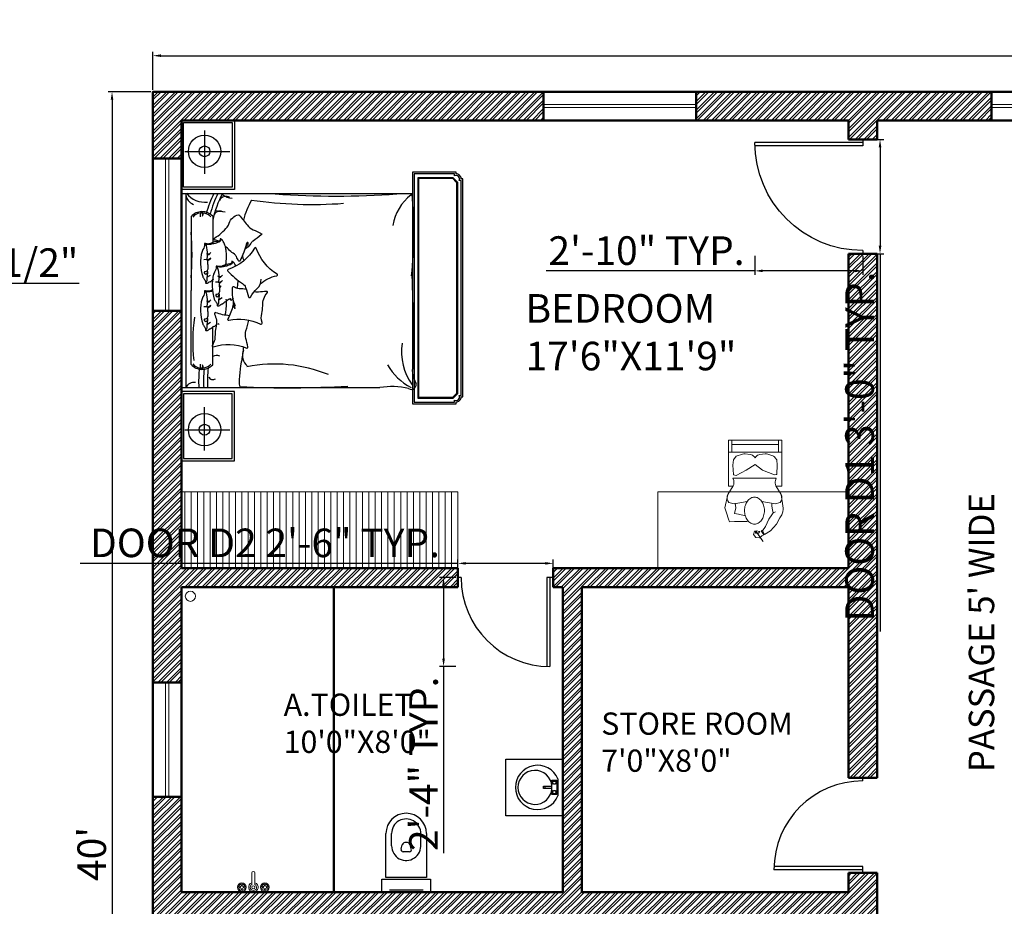
# Model space of a CAD drawing. Units: inches. Extents: x 3590 to 5167, y 65 to 1917.
# Tile 27 of 100: x 4378 to 4688, y 1549 to 1829. Entities that reach past the tile are written whole.
import ezdxf

# ---------------------------------------------------------------- set-up
doc = ezdxf.new("R2010")
doc.units = ezdxf.units.IN
for name, color, linetype, lineweight in [('A-ANNO-DIMS', 2, 'Continuous', 18), ('A-AREA-IDEN', 7, 'Continuous', 18), ('A-DOOR', 3, 'Continuous', 25), ('A-FLOR-FIXT', 8, 'Continuous', 18), ('A-FURN', 21, 'Continuous', 18), ('A-GLAZ', 4, 'Continuous', 18), ('A-WALL', 7, 'Continuous', 50), ('A-WALL-PATT', 251, 'Continuous', 13)]:
    doc.layers.add(name, color=color, linetype=linetype, lineweight=lineweight)
for name, color, linetype in [('FUR', 42, 'Continuous'), ('HA-FUR', 8, 'Continuous'), ('HA-P', 8, 'Continuous'), ('SAN', 5, 'Continuous'), ('SANTEH', 7, 'Continuous'), ('wood', 26, 'Continuous')]:
    doc.layers.add(name, color=color, linetype=linetype)
doc.styles.get("Standard").update_dxf_attribs({"font": 'arial.ttf'})
doc.dimstyles.new('ISO-25', dxfattribs={"dimtxt": 9, "dimasz": 2.5, "dimexe": 1.25, "dimexo": 0.625, "dimtad": 1, "dimdec": 1, "dimlunit": 3, "dimtxsty": 'Standard', "dimcen": 2.5, "dimadec": 0, "dimazin": 0, "dimtfac": 1, "dimtdec": 1, "dimtmove": 0, "dimatfit": 3, "dimfxl": 1, "dimarcsym": 0})

# ---------------------------------------------------------------- blocks, each defined once
blk = doc.blocks.new('*D101')
at = {"layer": 'A-ANNO-DIMS', "color": 0, "lineweight": -2, "transparency": 16777216}
for p, q in [((4420.27, 1806.62), (4420.27, 1818.61)), ((4422.77, 1817.36), (5077.77, 1817.36)), ((5080.27, 1806.62), (5080.27, 1818.61))]:
    blk.add_line(p, q, dxfattribs=at)
at = {"layer": 'A-ANNO-DIMS', "color": 0, "transparency": 16777216}
for points in [[(4422.77, 1817.78), (4422.77, 1816.95), (4420.27, 1817.36)], [(5077.77, 1817.78), (5077.77, 1816.95), (5080.27, 1817.36)]]:
    blk.add_solid(points, dxfattribs=at)
at = {"layer": 'Defpoints', "color": 0, "transparency": 16777216}
for p in [(5080.27, 1817.36), (4420.27, 1806), (5080.27, 1806)]:
    blk.add_point(p, dxfattribs=at)
at = {"layer": 'A-ANNO-DIMS', "color": 0, "transparency": 16777216, "insert": (4750.27, 1822.57), "char_height": 9, "attachment_point": 5}
blk.add_mtext("55'", dxfattribs=at)
blk = doc.blocks.new('*D102')
at = {"layer": 'A-ANNO-DIMS', "color": 0, "lineweight": -2, "transparency": 16777216}
for p, q in [((4419.65, 1806), (4406.15, 1806)), ((4407.4, 1803.5), (4407.4, 1328.5)), ((4419.65, 1326), (4406.15, 1326))]:
    blk.add_line(p, q, dxfattribs=at)
at = {"layer": 'A-ANNO-DIMS', "color": 0, "transparency": 16777216}
for points in [[(4406.98, 1803.5), (4407.82, 1803.5), (4407.4, 1806)], [(4406.98, 1328.5), (4407.82, 1328.5), (4407.4, 1326)]]:
    blk.add_solid(points, dxfattribs=at)
at = {"layer": 'Defpoints', "color": 0, "transparency": 16777216}
for p in [(4420.27, 1806), (4407.4, 1326), (4420.27, 1326)]:
    blk.add_point(p, dxfattribs=at)
at = {"layer": 'A-ANNO-DIMS', "color": 0, "transparency": 16777216, "insert": (4402.18, 1566), "char_height": 9, "attachment_point": 5, "rotation": 90}
blk.add_mtext("40'", dxfattribs=at)
blk = doc.blocks.new('D1')
for p, q in [((1, 0), (1, 34)), ((2, 0), (2, 33.99)), ((0, 0), (2, 0)), ((35, 0), (36, 0))]:
    blk.add_line(p, q)
at = {"ltscale": 0.5}
blk.add_arc((1, 0), 34, 0, 90, dxfattribs=at)
blk = doc.blocks.new('D2')
for p, q in [((1, 0), (1, 28)), ((2, 0), (2, 27.98)), ((0, 0), (2, 0)), ((29, 0), (30, 0))]:
    blk.add_line(p, q)
at = {"ltscale": 0.5}
blk.add_arc((1, 0), 28, 0, 90, dxfattribs=at)
blk = doc.blocks.new('Faucet - Bathroom top')
for p, q in [((-4.107, 0.125), (-4.375, 0.125)), ((-3.75, 0.4788), (-3.75, 0.75)), ((-3.5, 0.482), (-3.5, 0.75)), ((-3.1461, 0.125), (-2.875, 0.125)), ((3.143, 0.125), (2.875, 0.125)), ((3.5, 0.4788), (3.5, 0.75)), ((3.75, 0.482), (3.75, 0.75)), ((4.1039, 0.125), (4.375, 0.125)), ((-4.1039, -0.125), (-4.375, -0.125)), ((-3.75, -0.4821), (-3.75, -0.75)), ((-3.5, -0.4789), (-3.5, -0.75)), ((-3.143, -0.125), (-2.875, -0.125)), ((-0.5, -0.8639), (-0.5, -4.5)), ((0.5, -4.5), (0.5, -0.8631)), ((3.1461, -0.125), (2.875, -0.125)), ((3.5, -0.4821), (3.5, -0.75)), ((3.75, -0.4789), (3.75, -0.75)), ((4.107, -0.125), (4.375, -0.125))]:
    blk.add_line(p, q)
for centre, radius in [((-3.625, 0), 1.375), ((-4.625, 0), 0.2795), ((-3.625, 0), 0.5), ((-3.625, 1), 0.2795), ((-2.625, 0), 0.2795), ((0, 0), 0.5), ((3.625, 0), 1.375), ((2.625, 0), 0.2795), ((3.625, 0), 0.5), ((3.625, 1), 0.2795), ((4.625, 0), 0.2795), ((-3.625, -1), 0.2795), ((3.625, -1), 0.2795)]:
    blk.add_circle(centre, radius)
for centre, radius, start, end in [((-3.625, 0), 1, 105.2407, 164.2093), ((-3.625, 0), 1, 16.44125, 74.07887), ((0, 0), 1.5, 289.6514, 250.3603), ((0, 0), 1, 300.3431, 239.7554), ((3.625, 0), 1, 106.12, 164.0884), ((3.625, 0), 1, 16.23422, 73.90469), ((-3.625, 0), 1, 196.2342, 253.9047), ((-3.625, 0), 1, 286.12, 344.0884), ((3.625, 0), 1, 196.4413, 254.0789), ((3.625, 0), 1, 285.2407, 344.2093), ((0, -4.5), 0.5, 180, 0)]:
    blk.add_arc(centre, radius, start, end)
blk = doc.blocks.new('y3')
at = {"layer": 'SANTEH', "ltscale": 5}
for p, q in [((37.5, 130.7), (37.5, 520.7)), ((87.5, 410.7), (87.5, 520.7)), ((346.6, 426.1), (347.5, 520.7)), ((397.5, 520.7), (397.5, 130.7)), ((171.9, 384.5), (181.1, 421.3)), ((244.3, 357.8), (190.7, 357.8)), ((263.1, 384.5), (253.9, 421.3)), ((397.5, 130.7), (37.5, 130.7)), ((67.5, 20.7), (367.5, 20.7))]:
    blk.add_line(p, q, dxfattribs=at)
blk.add_lwpolyline([(0, 115), (435, 115), (435, 0), (0, 0), (0, 115)], dxfattribs=at)
for centre, radius, start, end in [((217.5, 520.7), 180, 0, 180), ((217.5, 520.7), 130, 359.15795, 180), ((217.5, 399.9), 42.2, 30.52342, 149.47658), ((217.5, 410.7), 130, 180, 5.98548), ((190.7, 377.8), 20, 160.50385, 270), ((244.3, 377.8), 20, 270, 19.49615)]:
    blk.add_arc(centre, radius, start, end, dxfattribs=at)
blk = doc.blocks.new('r11')
at = {"layer": 'SANTEH', "ltscale": 5}
for p, q in [((0, 0), (600, 0)), ((0, -600), (0, 0)), ((600, 0), (600, -600)), ((210, -50), (390, -50)), ((210, -50), (210, -50)), ((224, -63), (376, -63)), ((224, -113), (224, -63)), ((233, -79), (249, -69)), ((233, -98), (233, -79)), ((249, -107), (233, -98)), ((249, -69), (266, -79)), ((266, -98), (249, -107)), ((266, -79), (266, -98)), ((334, -79), (351, -69)), ((334, -98), (334, -79)), ((351, -107), (334, -98)), ((351, -69), (367, -79)), ((367, -98), (351, -107)), ((367, -79), (367, -98)), ((376, -63), (376, -113)), ((376, -113), (224, -113)), ((288, -202), (288, -113)), ((312, -184), (288, -184)), ((312, -202), (288, -202)), ((312, -113), (312, -202)), ((600, -600), (0, -600))]:
    blk.add_line(p, q, dxfattribs=at)
for centre, radius, start, end in [((300, -266), 234, 112.5, 67.5), ((300, -293), 180, 93.8183, 86.1817)]:
    blk.add_arc(centre, radius, start, end, dxfattribs=at)
blk = doc.blocks.new('A$C0A42580C')
at = {"layer": 'SAN'}
for p, q in [((0.2873, 0.0301), (0.2873, 0.4484)), ((2.8678, 0.0301), (2.8678, 0.4484)), ((0.0949, 0.2135), (0.4958, 0.2135)), ((3.0601, 0.2135), (2.6592, 0.2135))]:
    blk.add_line(p, q, dxfattribs=at)
for centre, radius in [((0.2873, 0.2135), 0.15), ((2.8678, 0.2135), 0.15), ((0.2873, 0.2135), 0.05), ((2.8678, 0.2135), 0.05)]:
    blk.add_circle(centre, radius, dxfattribs=at)
at = {"layer": 'wood'}
for p, q in [((0.6775, 0.8851), (0.6775, 2.1392)), ((2.4775, 0.8016), (2.4775, 1.838)), ((2.4775, 0), (2.4775, 0.8016)), ((1.6633, 0.3438), (1.6434, 0.3761)), ((0.888, 0.289), (1.1327, 0.289)), ((1.5, 0.3423), (1.5016, 0.3142)), ((2.267, 0.289), (1.9163, 0.289)), ((1.2906, 0.2348), (1.2921, 0.2067)), ((1.4538, 0.2362), (1.434, 0.2685)), ((1.7287, 0.2348), (1.7302, 0.2067)), ((1.8919, 0.2362), (1.8721, 0.2685)), ((0.6775, 0.039), (2.4775, 0.039)), ((0.8909, 0.089), (1.5775, 0.089)), ((2.2642, 0.089), (1.5775, 0.089)), ((0.6775, 0), (2.4775, 0))]:
    blk.add_line(p, q, dxfattribs=at)
blk.add_lwpolyline([(0.6775, 0), (0.6775, 0.8851)], dxfattribs=at)
for points in [[(1.516, 0.7294, -0.128392), (1.4401, 0.8834, 0.70791), (1.427, 0.8863, -0.16964), (1.1848, 0.6919, 0.664036), (1.184, 0.6776, -0.184649), (1.3819, 0.4332, 0.662242), (1.3969, 0.4309, 0.078539), (1.5137, 0.5669, -0.1736), (1.5484, 0.5947, -0.02159), (1.6357, 0.6205, 0.697276), (1.6379, 0.6405, -0.093019), (1.5606, 0.699, 0.216632), (1.4719, 0.7371, -2.511293)], [(1.1211, 0.3454, 0.032543), (1.1095, 0.3091, -0.658965), (1.0917, 0.3063, 0.074753), (0.9887, 0.4234, 0.100988), (0.953, 0.4429, -0.270711), (0.8753, 0.5273, -0.276825), (0.8775, 0.5337, -0.014937), (0.9701, 0.6081, 0.134834), (1.0135, 0.6643, -0.023706), (1.0474, 0.7372, -0.664036), (1.0616, 0.7394, -0.035987), (1.119, 0.6627, 0.118631), (1.1415, 0.6412, -0.132738), (1.1955, 0.5864)], [(1.6795, 0.4818, 0.263265), (1.7191, 0.4839, -0.026108), (1.743, 0.4973, 0.027613), (1.7137, 0.4764, -0.089259), (1.8403, 0.429, 0.662242), (1.8528, 0.4376, -0.162037), (1.8882, 0.732, 0.676499), (1.8733, 0.748, -0.160513), (1.7901, 0.7439, 0.07473), (1.7202, 0.7523, -0.187721), (1.5966, 0.7963, 0.70791), (1.5851, 0.7895, -0.010003), (1.5921, 0.7143, -0.07079), (1.5891, 0.6719, 0.099539)], [(1.1759, 0.5928, 0.013884), (1.1549, 0.6131, 0.174178), (1.1437, 0.6177, 0.104076), (1.1358, 0.6165, 0.389829), (1.1324, 0.6097, 0.296089), (1.1415, 0.6019, -0.036701), (1.1572, 0.5985, -0.040547), (1.3022, 0.543, -0.70791), (1.3021, 0.5296, -0.016811), (1.2631, 0.5085, 0.11866), (1.2414, 0.4904, -0.048791), (1.1649, 0.4055, 0.103757)], [(1.5674, 0.601, 0.057807), (1.5606, 0.5339, -0.173425), (1.5457, 0.49, 0.589988), (1.5538, 0.4706, 0.137312), (1.7236, 0.4985, 0.137312)], [(1.8113, 0.4446, -0.069098), (1.7831, 0.3187, 0.658965), (1.7961, 0.3062, -0.049789), (1.8516, 0.3234, -0.103757), (1.8905, 0.3233, 0.055725), (2.0203, 0.3103, -0.11866), (2.0478, 0.304, 0.016811), (2.0881, 0.2856, 0.70791), (2.0989, 0.2936, -0.16964), (2.1104, 0.604, 0.664036), (2.1001, 0.6139, 0.023706), (2.0214, 0.597, -0.134834), (1.9505, 0.5976, 0.012748), (1.8522, 0.6228)], [(1.3107, 0.4764, 0.145733), (1.3069, 0.4677, 0.488583), (1.3089, 0.4657, -0.012138), (1.3131, 0.4661, -0.125673), (1.3213, 0.4646, -0.750706)], [(1.3153, 0.4751, -0.274893), (1.3379, 0.4529, 0.051436), (1.3468, 0.4293, -0.086628), (1.3532, 0.4078, 0.040196), (1.3593, 0.3772, -0.184744), (1.3556, 0.3344, -2.554464)], [(1.317, 0.4683, -0.060098), (1.3283, 0.4571, -0.16247), (1.3313, 0.4487, 0.120018), (1.3493, 0.3815, -0.060072), (1.3541, 0.3695, -0.13107), (1.3541, 0.3395, -0.024415), (1.3534, 0.3373, 0.070398), (1.3503, 0.3233, 0.528689), (1.3524, 0.3216, -0.069388), (1.3557, 0.3222, -0.158233), (1.4075, 0.3065, 0.085461), (1.4255, 0.2981, 0.147196), (1.6571, 0.3041, 0.10985), (1.6823, 0.3191, -0.179095), (1.7126, 0.3319, -2.318897)], [(1.1013, 0.3688, 0.145733), (1.0975, 0.3601, 0.488583), (1.0995, 0.3581, -0.012138), (1.1036, 0.3585, -0.125673), (1.1119, 0.357, -0.750706)], [(1.1059, 0.3675, -0.274893), (1.1285, 0.3453, 0.051436), (1.1373, 0.3217, -0.086628), (1.1438, 0.3003, 0.040196), (1.1499, 0.2696, -0.184744), (1.1462, 0.2269, -2.554464)], [(1.4359, 0.3803, -0.198519), (1.452, 0.3494, 0.826402), (1.4558, 0.349, 0.095956), (1.4561, 0.3528, 0.242899), (1.4461, 0.3686, -17.523452)], [(1.5447, 0.3525, -0.083557), (1.507, 0.3546, 0.203162), (1.4851, 0.3792, -0.208037), (1.5043, 0.3409, 0.124669), (1.4432, 0.3469, 0.965934)], [(1.5394, 0.3688, 0.145733), (1.5356, 0.3601, 0.488583), (1.5376, 0.3581, -0.012138), (1.5418, 0.3585, -0.125673), (1.55, 0.357, -0.750706)], [(1.1076, 0.3607, -0.060098), (1.1189, 0.3495, -0.16247), (1.1219, 0.3411, 0.120018), (1.1399, 0.2739, -0.060072), (1.1447, 0.2619, -0.13107), (1.1447, 0.2319, -0.024415), (1.144, 0.2297, 0.070398), (1.1409, 0.2157, 0.528689), (1.143, 0.2141, -0.069388), (1.1463, 0.2146, -0.158233), (1.1981, 0.1989, 0.085461), (1.2161, 0.1905, 0.147196), (1.4477, 0.1965, 0.10985), (1.4728, 0.2115, -0.179095), (1.5032, 0.2244, -2.318897)], [(1.3509, 0.3219, -0.117141), (1.3688, 0.335, -0.025084), (1.4533, 0.348, 0.033691)], [(1.5447, 0.3525, -0.008229), (1.5728, 0.3519, 0.033691)], [(1.5721, 0.286, 0.022869), (1.578, 0.2739, -0.060072), (1.5828, 0.2619, -0.13107), (1.5828, 0.2319, -0.024415), (1.5821, 0.2297, 0.070398), (1.579, 0.2157, 0.528689), (1.5811, 0.2141, -0.069388), (1.5844, 0.2146, -0.158233), (1.6362, 0.1989, 0.085461), (1.6542, 0.1905, 0.147196), (1.8858, 0.1965, 0.10985), (1.911, 0.2115, -0.179095), (1.9413, 0.2244, -2.318897)], [(1.5728, 0.3519, -0.46905), (1.6152, 0.321, 0.420988), (1.62, 0.3169, 0.857652), (1.6221, 0.3484, 0.548526)], [(1.5838, 0.2873, 0.023398), (1.588, 0.2696, -0.184744), (1.5843, 0.2269, -2.554464)], [(1.603, 0.3451, -0.099719), (1.6221, 0.3484, 0.102691)], [(1.6214, 0.3487, -0.010168), (1.6558, 0.3447, 0.033691), (1.6907, 0.3423, -0.220869), (1.7148, 0.3311, -0.288972)], [(1.1415, 0.2143, -0.117141), (1.1594, 0.2274, -0.025084), (1.2439, 0.2405, 0.033691)], [(1.2265, 0.2728, -0.198519), (1.2426, 0.2418, 0.826402), (1.2463, 0.2415, 0.095956), (1.2467, 0.2452, 0.242899), (1.2366, 0.2611, -17.523452)], [(1.3353, 0.2449, -0.083557), (1.2976, 0.247, 0.203162), (1.2757, 0.2717, -0.208037), (1.2948, 0.2333, 0.124669), (1.2338, 0.2393, 0.965934)], [(1.3353, 0.2449, -0.008229), (1.3633, 0.2443, 0.033691)], [(1.3633, 0.2443, -0.46905), (1.4058, 0.2134, 0.420988), (1.4106, 0.2093, 0.857652), (1.4127, 0.2408, 0.548526)], [(1.3936, 0.2375, -0.099719), (1.4127, 0.2408, 0.102691)], [(1.412, 0.2411, -0.010168), (1.4464, 0.2371, 0.033691), (1.4812, 0.2348, -0.220869), (1.5054, 0.2235, -0.288972)], [(1.5796, 0.2143, -0.117141), (1.5975, 0.2274, -0.025084), (1.682, 0.2405, 0.033691)], [(1.6646, 0.2728, -0.198519), (1.6807, 0.2418, 0.826402), (1.6845, 0.2415, 0.095956), (1.6848, 0.2452, 0.242899), (1.6748, 0.2611, -17.523452)], [(1.7734, 0.2449, -0.083557), (1.7357, 0.247, 0.203162), (1.7138, 0.2717, -0.208037), (1.733, 0.2333, 0.124669), (1.6719, 0.2393, 0.965934)], [(1.7734, 0.2449, -0.008229), (1.8015, 0.2443, 0.033691)], [(1.8015, 0.2443, -0.46905), (1.8439, 0.2134, 0.420988), (1.8487, 0.2093, 0.857652), (1.8508, 0.2408, 0.548526)], [(1.8317, 0.2375, -0.099719), (1.8508, 0.2408, 0.102691)], [(1.8501, 0.2411, -0.010168), (1.8845, 0.2371, 0.033691), (1.9193, 0.2348, -0.220869), (1.9435, 0.2235, -0.288972)]]:
    blk.add_lwpolyline(points, format="xyb", dxfattribs=at)
for points in [[(0.64, 0), (0, 0), (0, 0.49), (0.64, 0.49)], [(0.62, 0.02), (0.02, 0.02), (0.02, 0.47), (0.62, 0.47)], [(2.515, 0), (3.155, 0), (3.155, 0.49), (2.515, 0.49)], [(2.535, 0.02), (3.135, 0.02), (3.135, 0.47), (2.535, 0.47)]]:
    blk.add_lwpolyline(points, close=True, dxfattribs=at)
for centre, radius, start, end in [((1.0344, -2.14), 4.292, 84.56078, 94.7164), ((1.0494, 2.4026), 0.4515, 217.47941, 260.35986), ((2.0208, -11.0786), 13.2288, 88.75549, 92.51133), ((2.1491, 2.5471), 0.5083, 260.65485, 306.44155), ((2.3125, 2.3833), 0.2443, 254.1515, 300.95574), ((2.0168, 2.3573), 0.5127, 299.08175, 333.44367), ((2.4501, 2.1309), 0.0445, 324.18954, 118.92203), ((3.1371, 1.9502), 0.669, 166.6404, 189.65708), ((-7.0839, 1.4328), 7.7858, 355.84817, 4.15183), ((-3.167, 1.2143), 3.9465, 351.77286, 4.18386), ((-7.2439, 0.9937), 9.7233, 357.34474, 3.23068), ((3.5803, 0.8622), 1.3213, 157.81295, 191.15154), ((1.1611, 1.4181), 0.8768, 241.21362, 254.41879), ((1.2583, 0.6364), 0.0695, 238.58923, 301.92671), ((1.7861, -2.1601), 2.7557, 80.89877, 83.46656), ((2.181, 0.6859), 0.1221, 247.37754, 321.13165), ((2.4192, 1.3819), 0.8461, 255.77539, 273.25587), ((0.5904, 0.4689), 0.13, 317.38218, 359.70393), ((1.3546, 0.4469), 0.0529, 114.21284, 146.15395), ((2.6126, -2.3504), 3.1201, 113.83178, 114.21284), ((1.4714, 0.0722), 0.4528, 80.62397, 88.74059), ((1.4035, -0.3388), 0.8693, 79.71489, 80.62397), ((1.6301, 0.4539), 0.0342, 31.14095, 54.95422), ((1.6709, 0.4489), 0.0156, 131.9623, 212.08127), ((1.5664, 0.4154), 0.1086, 24.20989, 31.14095), ((1.6627, 0.4587), 0.00309, 275.52245, 24.20989), ((1.1611, 1.3191), 1.0568, 242.76671, 257.10398), ((0.7723, 0.4131), 0.0674, 147.68233, 245.79865), ((0.0312, 0.4583), 0.8174, 350.42368, 356.2506), ((0.9021, 0.3562), 0.0605, 155.8342, 254.41058), ((1.1452, 0.3394), 0.0529, 114.21284, 146.15395), ((2.4032, -2.458), 3.1201, 113.55686, 114.21284), ((1.2046, 0.2912), 0.121, 99.42032, 113.55686), ((1.2774, -0.1478), 0.5659, 95.90379, 99.42032), ((1.2626, -0.005), 0.4223, 88.74059, 95.90379), ((1.2619, -0.0354), 0.4528, 80.62397, 88.74059), ((1.1941, -0.4464), 0.8693, 79.45871, 80.62397), ((1.4207, 0.3463), 0.0342, 31.14095, 54.95422), ((1.6729, 0.4422), 0.0178, 140.41793, 157.63267), ((1.7007, -0.005), 0.4223, 88.74059, 95.90379), ((1.7235, 0.4818), 0.0777, 212.08127, 227.364), ((1.6635, 0.4499), 0.00568, 95.52245, 140.41793), ((1.6391, 0.3902), 0.0469, 17.32618, 47.364), ((1.7106, 0.4125), 0.028, 197.32618, 226.17302), ((1.6431, 0.3422), 0.0695, 26.61764, 46.17302), ((1.8202, 0.431), 0.1287, 206.61764, 215.96192), ((1.7001, -0.0354), 0.4528, 80.62397, 88.74059), ((1.6322, -0.4464), 0.8693, 78.43923, 80.62397), ((1.1611, 1.3191), 1.0937, 243.75553, 254.4906), ((1.1611, 1.2816), 1.0937, 243.75553, 254.38927), ((0.9846, 0.1903), 0.1381, 134.39284, 227.23745), ((1.4614, 0.3413), 0.0156, 131.9623, 212.08127), ((1.4635, 0.3347), 0.0178, 140.41793, 157.63267), ((1.4541, 0.3424), 0.00568, 95.52245, 140.41793), ((1.357, 0.3078), 0.1086, 24.20989, 31.14095), ((1.4533, 0.3511), 0.00309, 275.52245, 24.20989), ((1.5012, 0.305), 0.028, 197.32618, 226.17302), ((1.4337, 0.2347), 0.0695, 26.61764, 46.17302), ((1.715, 0.3349), 0.00379, 207.1817, 328.02977), ((1.6975, 0.3419), 0.023, 350.76434, 35.96192), ((1.7058, 0.3406), 0.0145, 328.02977, 350.76434), ((1.9016, 0.3347), 0.0178, 140.41793, 157.63267), ((1.9522, 0.3743), 0.0777, 212.08127, 227.364), ((1.8922, 0.3424), 0.00568, 95.52245, 140.41793), ((1.8678, 0.2827), 0.0469, 17.32618, 47.364), ((1.9393, 0.305), 0.028, 197.32618, 226.17302), ((1.8718, 0.2347), 0.0695, 26.61764, 46.17302), ((2.2511, 0.3256), 0.071, 155.86842, 211.04513), ((2.1704, 0.1903), 0.1381, 312.76255, 45.60716), ((2.3616, 0.2915), 0.0419, 290.78583, 35.36309), ((0.5293, 0.2241), 0.2307, 309.63048, 4.27465), ((0.8396, 0.185), 0.0112, 314.89662, 45.10338), ((0.8413, 0.1846), 0.0128, 299.47062, 57.44416), ((0.8844, 0.2286), 0.0569, 229.70587, 281.11527), ((0.8802, 0.1371), 0.0592, 81.47786, 123.11925), ((0.8698, 0.1793), 0.0229, 77.14902, 159.1786), ((0.9986, 0.1735), 0.1427, 136.58239, 164.9725), ((1.6108, 0.3235), 0.1287, 206.61764, 215.96192), ((1.5055, 0.2273), 0.00379, 207.1817, 328.02977), ((1.4881, 0.2344), 0.023, 350.76434, 35.96192), ((1.4964, 0.233), 0.0145, 328.02977, 350.76434), ((2.0489, 0.3235), 0.1287, 206.61764, 215.96192), ((1.9436, 0.2273), 0.00379, 207.1817, 328.02977), ((1.9262, 0.2344), 0.023, 350.76434, 35.96192), ((1.9345, 0.233), 0.0145, 328.02977, 350.76434), ((2.2706, 0.2286), 0.0569, 258.88473, 310.29413), ((2.1565, 0.1735), 0.1427, 15.0275, 43.41761), ((2.2749, 0.1371), 0.0592, 56.88075, 98.52214), ((2.2853, 0.1793), 0.0229, 20.8214, 102.85098), ((2.4192, 1.2667), 1.0261, 263.09035, 273.25587), ((2.3138, 0.1846), 0.0128, 122.55584, 240.52938), ((2.3154, 0.185), 0.0112, 134.89662, 225.10338), ((2.4192, 1.2667), 1.0629, 263.94374, 273.25587), ((0.6729, 0.151), 0.1135, 279.23824, 338.73819), ((0.9466, 0.1765), 0.0862, 185.53723, 234.68694), ((1.2481, -2.5919), 2.6893, 85.4722, 94.5278), ((2.0447, 1.7022), 1.5979, 262.13639, 276.48786), ((2.2085, 0.1765), 0.0862, 305.31306, 354.46277), ((2.4192, 1.2218), 1.0629, 263.23622, 273.25587), ((2.508, 0.1152), 0.0792, 169.94668, 248.24015)]:
    blk.add_arc(centre, radius, start, end, dxfattribs=at)
blk = doc.blocks.new('A$C623F1DA0')
at = {"layer": 'FUR'}
blk.add_lwpolyline([(0.628, 2.912, 0.414214), (0.562, 2.978), (0.562, 3), (0, 3), (0, 0), (0.562, 0), (0.562, 0.022, 0.414214), (0.628, 0.088), (0.65, 0.088), (0.65, 2.912)], format="xyb", close=True, dxfattribs=at)
at = {"layer": 'HA-FUR'}
blk.add_lwpolyline([(0.603, 2.892, 0.710288), (0.542, 2.953), (0.542, 2.98), (0.02, 2.98), (0.02, 0.02), (0.542, 0.02), (0.542, 0.047, 0.710288), (0.603, 0.108), (0.63, 0.108), (0.63, 2.892)], format="xyb", close=True, dxfattribs=at)
at = {"layer": 'HA-P'}
for points in [[(0.07, 2.93), (0.521, 2.93), (0.58, 2.871), (0.58, 0.129), (0.521, 0.07), (0.07, 0.07)], [(0.08, 2.92), (0.517, 2.92), (0.57, 2.867), (0.57, 0.133), (0.517, 0.08), (0.08, 0.08)]]:
    blk.add_lwpolyline(points, close=True, dxfattribs=at)
blk = doc.blocks.new('DESK-CHAIR')
for p, q in [((3674.9, 1522.4), (3674.54, 1520.79)), ((3675.51, 1522.74), (3674.9, 1522.4)), ((3680.2, 1521.08), (3677.49, 1522.71)), ((3694.59, 1522.58), (3680.09, 1522.58)), ((3680.09, 1522.58), (3680.09, 1521.15)), ((3694.59, 1505.74), (3694.59, 1522.58)), ((3674.54, 1520.79), (3675.25, 1516.67)), ((3682.6, 1521.15), (3681.85, 1520.9)), ((3682.6, 1521.15), (3682.6, 1507.53)), ((3682.6, 1507.53), (3682.6, 1521.15)), ((3683.49, 1520.07), (3683.66, 1520.91)), ((3685.1, 1517.02), (3683.49, 1520.07)), ((3683.73, 1520.97), (3686.72, 1521.15)), ((3686.72, 1521.15), (3688.33, 1520.97)), ((3688.33, 1520.97), (3689.58, 1520.07)), ((3689.58, 1520.07), (3690.17, 1518.15)), ((3686.89, 1514.16), (3685.1, 1517.02)), ((3690.24, 1517.32), (3690.04, 1515.67)), ((3685.1, 1511.83), (3686.89, 1514.16)), ((3689.31, 1514.37), (3689.04, 1514.16)), ((3689.31, 1513.95), (3689.04, 1514.16)), ((3690.24, 1511), (3690.04, 1512.64)), ((3664.74, 1511.43), (3666.04, 1512.26)), ((3665.07, 1511.29), (3664.74, 1511.43)), ((3664.84, 1511.19), (3666.07, 1511.86)), ((3666.04, 1509.36), (3664.84, 1511.19)), ((3666.04, 1512.26), (3666.24, 1511.79)), ((3666.07, 1511.86), (3667.43, 1510.93)), ((3667.43, 1510.93), (3669.7, 1509.83)), ((3669.7, 1509.83), (3671.06, 1508.9)), ((3674.54, 1507.89), (3675.25, 1512.01)), ((3683.67, 1508.07), (3685.1, 1511.83)), ((3689.78, 1508.89), (3690.17, 1510.17)), ((3668.13, 1507.37), (3666.04, 1509.36)), ((3670.06, 1506.4), (3668.13, 1507.37)), ((3671.06, 1508.9), (3671.66, 1508.47)), ((3671.66, 1508.47), (3671.96, 1507.77)), ((3674.9, 1506.27), (3674.54, 1507.89)), ((3680.2, 1507.6), (3677.49, 1505.97)), ((3680.09, 1507.53), (3680.09, 1505.74)), ((3682.6, 1507.53), (3681.85, 1507.78)), ((3683.8, 1507.4), (3683.67, 1508.07)), ((3683.88, 1507.34), (3686.72, 1507.17)), ((3686.72, 1507.17), (3688.33, 1507.35)), ((3688.33, 1507.35), (3689.03, 1507.86)), ((3677.49, 1505.97), (3673.14, 1505.31)), ((3675.51, 1505.94), (3674.9, 1506.27)), ((3680.09, 1505.74), (3694.59, 1505.74))]:
    blk.add_line(p, q)
for points in [[(3677.49, 1522.71), (3673.28, 1523.65), (3671.67, 1523.12), (3669.7, 1522.58), (3668.81, 1522.22), (3668.99, 1520.61), (3668.99, 1519), (3668.99, 1516.67)], [(3664.74, 1511.43), (3664.42, 1512.05), (3663.77, 1512.78), (3663.87, 1513.9), (3664.88, 1514.67), (3665.92, 1514.37), (3665.9, 1514.02), (3665.32, 1514.02), (3665.3, 1513.1), (3665.82, 1512.66), (3666.07, 1513.84)], [(3671.66, 1508.47), (3672.6, 1508.69), (3673.82, 1508.93), (3674.7, 1508.93)], [(3670.06, 1506.4), (3671.04, 1505.75), (3672.02, 1505.46), (3672.8, 1505.31), (3673.24, 1505.31)]]:
    blk.add_lwpolyline(points)
at = {"const_width": 0.39}
blk.add_lwpolyline([(3666.01, 1513.98), (3662.61, 1511.61)], dxfattribs=at)
for centre, radius, start, end in [((3676.47, 1521), 1.98, 59.0235, 119.0669), ((3681.22, 1522.78), 1.98, 239.0235, 288.4436), ((3683.74, 1520.89), 0.0779, 93.3682, 168.6956), ((3683.74, 1520.89), 0.0779, 93.3682, 168.6956), ((3688.27, 1517.56), 1.98, 352.8785, 17.0946), ((3688.07, 1515.92), 1.98, 308.6739, 352.8785), ((3688.07, 1512.4), 1.98, 7.1215, 51.3261), ((3688.27, 1510.75), 1.98, 342.9054, 7.1215), ((3681.22, 1505.89), 1.98, 71.5564, 120.9765), ((3683.88, 1507.42), 0.0779, 191.3044, 266.6318), ((3687.88, 1509.47), 1.98, 305.5514, 342.9054), ((3676.47, 1507.67), 1.98, 240.9331, 300.9765)]:
    blk.add_arc(centre, radius, start, end)
blk = doc.blocks.new('*D312')
at = {"layer": 'A-ANNO-DIMS', "color": 0, "lineweight": -2, "transparency": 16777216}
for p, q in [((4644.4, 1791), (4650.42, 1791)), ((4649.17, 1788.5), (4649.17, 1757.5)), ((4644.4, 1755), (4650.42, 1755)), ((4649.17, 1755), (4649.17, 1636.06))]:
    blk.add_line(p, q, dxfattribs=at)
at = {"layer": 'A-ANNO-DIMS', "color": 0, "transparency": 16777216}
for points in [[(4648.76, 1788.5), (4649.59, 1788.5), (4649.17, 1791)], [(4648.76, 1757.5), (4649.59, 1757.5), (4649.17, 1755)]]:
    blk.add_solid(points, dxfattribs=at)
at = {"layer": 'Defpoints', "color": 0, "transparency": 16777216}
for p in [(4643.77, 1791), (4643.77, 1755), (4649.17, 1755)]:
    blk.add_point(p, dxfattribs=at)
at = {"layer": 'A-ANNO-DIMS', "color": 0, "transparency": 16777216, "insert": (4643.89, 1694.28), "char_height": 9, "attachment_point": 5, "rotation": 90}
blk.add_mtext('DOOR D1 3\'-0" TYP.', dxfattribs=at)
blk = doc.blocks.new('*D313')
at = {"layer": 'A-ANNO-DIMS', "color": 0, "lineweight": -2, "transparency": 16777216}
for p, q in [((4609.77, 1754.37), (4609.77, 1748.35)), ((4643.77, 1754.37), (4643.77, 1748.35)), ((4609.77, 1749.6), (4544.02, 1749.6)), ((4641.27, 1749.6), (4612.27, 1749.6))]:
    blk.add_line(p, q, dxfattribs=at)
at = {"layer": 'A-ANNO-DIMS', "color": 0, "transparency": 16777216}
for points in [[(4612.27, 1750.02), (4612.27, 1749.18), (4609.77, 1749.6)], [(4641.27, 1750.02), (4641.27, 1749.18), (4643.77, 1749.6)]]:
    blk.add_solid(points, dxfattribs=at)
at = {"layer": 'Defpoints', "color": 0, "transparency": 16777216}
for p in [(4609.77, 1755), (4643.77, 1755), (4609.77, 1749.6)]:
    blk.add_point(p, dxfattribs=at)
at = {"layer": 'A-ANNO-DIMS', "color": 0, "transparency": 16777216, "insert": (4575.65, 1754.82), "char_height": 9, "attachment_point": 5}
blk.add_mtext('2\'-10" TYP.', dxfattribs=at)
blk = doc.blocks.new('*D314')
at = {"layer": 'A-ANNO-DIMS', "color": 0, "lineweight": -2, "transparency": 16777216}
for p, q in [((4516.27, 1653.62), (4516.27, 1658.75)), ((4546.27, 1653.62), (4546.27, 1658.75)), ((4516.27, 1657.5), (4397.34, 1657.5)), ((4543.77, 1657.5), (4518.77, 1657.5))]:
    blk.add_line(p, q, dxfattribs=at)
at = {"layer": 'A-ANNO-DIMS', "color": 0, "transparency": 16777216}
for points in [[(4518.77, 1657.92), (4518.77, 1657.08), (4516.27, 1657.5)], [(4543.77, 1657.92), (4543.77, 1657.08), (4546.27, 1657.5)]]:
    blk.add_solid(points, dxfattribs=at)
at = {"layer": 'Defpoints', "color": 0, "transparency": 16777216}
for p in [(4516.27, 1657.5), (4516.27, 1653), (4546.27, 1653)]:
    blk.add_point(p, dxfattribs=at)
at = {"layer": 'A-ANNO-DIMS', "color": 0, "transparency": 16777216, "insert": (4455.55, 1662.78), "char_height": 9, "attachment_point": 5}
blk.add_mtext('DOOR D2 2\'-6" TYP.', dxfattribs=at)
blk = doc.blocks.new('*D315')
at = {"layer": 'A-ANNO-DIMS', "color": 0, "lineweight": -2, "transparency": 16777216}
for p, q in [((4515.65, 1653), (4510.52, 1653)), ((4511.77, 1650.5), (4511.77, 1627.5)), ((4515.65, 1625), (4510.52, 1625)), ((4511.77, 1625), (4511.77, 1566.24))]:
    blk.add_line(p, q, dxfattribs=at)
at = {"layer": 'A-ANNO-DIMS', "color": 0, "transparency": 16777216}
for points in [[(4511.36, 1650.5), (4512.19, 1650.5), (4511.77, 1653)], [(4511.36, 1627.5), (4512.19, 1627.5), (4511.77, 1625)]]:
    blk.add_solid(points, dxfattribs=at)
at = {"layer": 'Defpoints', "color": 0, "transparency": 16777216}
for p in [(4516.27, 1653), (4511.77, 1625), (4516.27, 1625)]:
    blk.add_point(p, dxfattribs=at)
at = {"layer": 'A-ANNO-DIMS', "color": 0, "transparency": 16777216, "insert": (4506.63, 1594.37), "char_height": 9, "attachment_point": 5, "rotation": 90}
blk.add_mtext('2\'-4" TYP.', dxfattribs=at)
blk = doc.blocks.new('*D320')
at = {"layer": 'A-ANNO-DIMS', "color": 0, "lineweight": -2, "transparency": 16777216}
for p, q in [((4247.49, 1753.73), (4247.49, 1744.5)), ((4304.85, 1753.73), (4304.85, 1744.5)), ((4249.99, 1745.75), (4302.35, 1745.75)), ((4304.85, 1745.75), (4397.07, 1745.75))]:
    blk.add_line(p, q, dxfattribs=at)
at = {"layer": 'A-ANNO-DIMS', "color": 0, "transparency": 16777216}
for points in [[(4249.99, 1746.17), (4249.99, 1745.33), (4247.49, 1745.75)], [(4302.35, 1746.17), (4302.35, 1745.33), (4304.85, 1745.75)]]:
    blk.add_solid(points, dxfattribs=at)
at = {"layer": 'Defpoints', "color": 0, "transparency": 16777216}
for p in [(4247.49, 1754.35), (4304.85, 1754.35), (4304.85, 1745.75)]:
    blk.add_point(p, dxfattribs=at)
at = {"layer": 'A-ANNO-DIMS', "color": 0, "transparency": 16777216, "insert": (4352.21, 1751.03), "char_height": 9, "attachment_point": 5}
blk.add_mtext('PLANT 4\'-9 1/2"', dxfattribs=at)

msp = doc.modelspace()

# ---------------------------------------------------------------- hatches: boundary and pattern name
at = {"layer": 'A-WALL-PATT', "transparency": 33554687}
h = msp.add_hatch(dxfattribs=at)
h.set_pattern_fill('ANSI32', color=256, scale=0.2)
h.paths.add_polyline_path([(4684.27, 1806), (4591.27, 1806), (4591.27, 1797), (4639.27, 1797), (4639.27, 1791), (4648.27, 1791), (4648.27, 1797), (4684.27, 1797)])
h.paths.add_polyline_path([(4543.27, 1806), (4420.27, 1806), (4420.27, 1785), (4429.27, 1785), (4429.27, 1797), (4445.92, 1797), (4543.27, 1797)])
h.paths.add_polyline_path([(4828.27, 1806), (4744.27, 1806), (4744.27, 1797), (4828.27, 1797)])
h.paths.add_polyline_path([(4648.27, 1755), (4639.27, 1755), (4639.27, 1656), (4546.27, 1656), (4546.27, 1650), (4549.27, 1650), (4549.27, 1554), (4429.27, 1554), (4429.27, 1584), (4420.27, 1584), (4420.27, 1539), (4429.27, 1539), (4429.27, 1545), (4639.27, 1545), (4639.27, 1539), (4648.27, 1539), (4648.27, 1560), (4639.27, 1560), (4639.27, 1554), (4555.27, 1554), (4555.27, 1650), (4639.27, 1650), (4639.27, 1590), (4648.27, 1590)])
h.paths.add_polyline_path([(4516.27, 1656), (4429.27, 1656), (4429.27, 1737), (4420.27, 1737), (4420.27, 1620), (4429.27, 1620), (4429.27, 1650), (4516.27, 1650)], flags=17)
h.paths.add_polyline_path([(5080.27, 1806), (4888.27, 1806), (4888.27, 1797), (4924.27, 1797), (4924.27, 1755), (4933.27, 1755), (4933.27, 1797), (5071.27, 1797), (5071.27, 1335), (4933.27, 1335), (4933.27, 1566), (4924.27, 1566), (4924.27, 1335), (4898.77, 1335), (4898.77, 1326), (5080.27, 1326)])
h.paths.add_polyline_path([(4933.27, 1719), (4924.27, 1719), (4924.27, 1638), (4933.27, 1638)], flags=17)
h.paths.add_polyline_path([(4802.77, 1335), (4777.27, 1335), (4777.27, 1503), (4756.27, 1503), (4756.27, 1494), (4768.27, 1494), (4768.27, 1431), (4696.27, 1431), (4696.27, 1494), (4708.27, 1494), (4708.27, 1503), (4639.27, 1503), (4639.27, 1494), (4687.27, 1494), (4687.27, 1431), (4681.27, 1431), (4681.27, 1422), (4768.27, 1422), (4768.27, 1335), (4726.27, 1335), (4726.27, 1326), (4802.77, 1326)])
h.paths.add_polyline_path([(4690.27, 1335), (4648.27, 1335), (4648.27, 1352.87), (4648.27, 1422), (4651.27, 1422), (4651.27, 1431), (4639.27, 1431), (4639.27, 1335), (4633.27, 1335), (4633.27, 1326), (4690.27, 1326)])
h.paths.add_polyline_path([(4585.27, 1335), (4584.72, 1335), (4429.27, 1335), (4429.27, 1491), (4420.27, 1491), (4420.27, 1326), (4585.27, 1326)])

# ---------------------------------------------------------------- linework, layer by layer
at = {"layer": 'A-FLOR-FIXT'}
msp.add_circle((4432.07, 1647.13), 1.6, dxfattribs=at)
at = {"layer": 'A-FURN'}
for p, q in [((4602.57, 1692.55), (4602.57, 1696.31)), ((4617.16, 1692.55), (4617.16, 1696.31)), ((4618.26, 1692.55), (4601.42, 1692.55)), ((4617.16, 1694.88), (4602.57, 1694.88)), ((4429.27, 1680), (4516.27, 1680)), ((4430.27, 1680), (4430.27, 1656)), ((4432.27, 1680), (4432.27, 1656)), ((4434.27, 1680), (4434.27, 1656)), ((4436.27, 1680), (4436.27, 1656)), ((4438.27, 1680), (4438.27, 1656)), ((4440.27, 1680), (4440.27, 1656)), ((4442.27, 1680), (4442.27, 1656)), ((4444.27, 1680), (4444.27, 1656)), ((4446.27, 1680), (4446.27, 1656)), ((4448.27, 1680), (4448.27, 1656)), ((4450.27, 1680), (4450.27, 1656)), ((4452.27, 1680), (4452.27, 1656)), ((4454.27, 1680), (4454.27, 1656)), ((4456.27, 1680), (4456.27, 1656)), ((4458.27, 1680), (4458.27, 1656)), ((4460.27, 1680), (4460.27, 1656)), ((4462.27, 1680), (4462.27, 1656)), ((4464.27, 1680), (4464.27, 1656)), ((4466.27, 1680), (4466.27, 1656)), ((4468.27, 1680), (4468.27, 1656)), ((4470.27, 1680), (4470.27, 1656)), ((4472.27, 1680), (4472.27, 1656)), ((4474.27, 1680), (4474.27, 1656)), ((4476.27, 1680), (4476.27, 1656)), ((4478.27, 1680), (4478.27, 1656)), ((4480.27, 1680), (4480.27, 1656)), ((4482.27, 1680), (4482.27, 1656)), ((4484.27, 1680), (4484.27, 1656)), ((4486.27, 1680), (4486.27, 1656)), ((4488.27, 1680), (4488.27, 1656)), ((4490.27, 1680), (4490.27, 1656)), ((4492.27, 1680), (4492.27, 1656)), ((4494.27, 1680), (4494.27, 1656)), ((4496.27, 1680), (4496.27, 1656)), ((4498.27, 1680), (4498.27, 1656)), ((4500.27, 1680), (4500.27, 1656)), ((4502.27, 1680), (4502.27, 1656)), ((4504.27, 1680), (4504.27, 1656)), ((4506.27, 1680), (4506.27, 1656)), ((4508.27, 1680), (4508.27, 1656)), ((4510.27, 1680), (4510.27, 1656)), ((4512.27, 1680), (4512.27, 1656)), ((4514.27, 1680), (4514.27, 1656)), ((4516.27, 1680), (4516.27, 1656)), ((4579.23, 1680), (4639.27, 1680)), ((4579.23, 1680), (4579.23, 1656))]:
    msp.add_line(p, q, dxfattribs=at)
msp.add_lwpolyline([(4612.77, 1674.11, 0.07405), (4612.52, 1675.79, 0.084801), (4611.86, 1677.11, 0.106336), (4610.79, 1678.06, 0.128955), (4609.65, 1678.36, 0.128955), (4608.5, 1678.06, 0.106336), (4607.44, 1677.11, 0.084801), (4606.77, 1675.79, 0.07405), (4606.52, 1674.11, 0.07405), (4606.77, 1672.43, 0.084801), (4607.44, 1671.11, 0.106336), (4608.5, 1670.16, 0.128955), (4609.65, 1669.86, 0.128955), (4610.79, 1670.16, 0.106336), (4611.86, 1671.11, 0.084801), (4612.52, 1672.43, 0.07405)], format="xyb", close=True, dxfattribs=at)
msp.add_lwpolyline([(4606.79, 1672.5), (4604.64, 1673.03), (4603.39, 1673.21), (4603.75, 1675), (4603.57, 1676.44)], dxfattribs=at)
at = {"layer": 'A-GLAZ'}
for p, q in [((4591.27, 1802), (4543.27, 1802)), ((4591.27, 1801), (4543.27, 1801)), ((4744.27, 1802), (4684.27, 1802)), ((4744.27, 1801), (4684.27, 1801)), ((4424.27, 1737), (4424.27, 1785)), ((4425.27, 1737), (4425.27, 1785)), ((4424.27, 1584), (4424.27, 1620)), ((4425.27, 1584), (4425.27, 1620))]:
    msp.add_line(p, q, dxfattribs=at)
at = {"layer": 'A-WALL'}
for p, q in [((4543.27, 1797), (4543.27, 1806)), ((4591.27, 1797), (4591.27, 1806)), ((4684.27, 1797), (4684.27, 1806)), ((4429.27, 1797), (4639.27, 1797)), ((4429.27, 1656), (4429.27, 1797)), ((4639.27, 1791), (4639.27, 1797)), ((4648.27, 1797), (4924.27, 1797)), ((4648.27, 1791), (4648.27, 1797)), ((4639.27, 1791), (4648.27, 1791)), ((4429.27, 1785), (4420.27, 1785)), ((4639.27, 1755), (4648.27, 1755)), ((4639.27, 1656), (4639.27, 1755)), ((4648.27, 1590), (4648.27, 1755)), ((4429.27, 1737), (4420.27, 1737)), ((4429.27, 1656), (4516.27, 1656)), ((4516.27, 1650), (4516.27, 1656)), ((4546.27, 1656), (4639.27, 1656)), ((4546.27, 1650), (4546.27, 1656)), ((4429.27, 1650), (4516.27, 1650)), ((4429.27, 1554), (4429.27, 1650)), ((4477.27, 1554), (4477.27, 1650)), ((4546.27, 1650), (4549.27, 1650)), ((4549.27, 1554), (4549.27, 1650)), ((4555.27, 1650), (4639.27, 1650)), ((4555.27, 1554), (4555.27, 1650)), ((4639.27, 1590), (4639.27, 1650)), ((4429.27, 1620), (4420.27, 1620)), ((4648.27, 1590), (4639.27, 1590)), ((4429.27, 1584), (4420.27, 1584)), ((4639.27, 1554), (4639.27, 1560)), ((4648.27, 1560), (4639.27, 1560)), ((4648.27, 1539), (4648.27, 1560)), ((4549.27, 1554), (4429.27, 1554)), ((4639.27, 1554), (4555.27, 1554))]:
    msp.add_line(p, q, dxfattribs=at)
msp.add_lwpolyline([(5080.27, 1806), (5080.27, 1326), (4420.27, 1326), (4420.27, 1806)], close=True, dxfattribs=at)

# ---------------------------------------------------------------- block references
at = {"layer": 'A-DOOR', "xscale": -1, "rotation": 90}
msp.add_blockref('D1', (4643.77, 1791), dxfattribs=at)
at = {"layer": 'A-DOOR'}
for p, rotation in [((4546.27, 1653), 180), ((4643.77, 1560), 89.99999999999999)]:
    msp.add_blockref('D2', p, dxfattribs=dict(at, rotation=rotation))
at = {"layer": 'A-FLOR-FIXT', "xscale": 0.0297800069284724, "yscale": 0.0297800069284724, "zscale": 0.0297800069284724, "rotation": 270}
msp.add_blockref('r11', (4549.27, 1595.88), dxfattribs=at)
at = {"layer": 'A-FLOR-FIXT', "xscale": 0.0353848906415677, "yscale": 0.0353848906415677, "zscale": 0.0353848906415677}
msp.add_blockref('y3', (4492.31, 1554), dxfattribs=at)
at = {"layer": 'A-FLOR-FIXT', "xscale": -1, "rotation": 180}
msp.add_blockref('Faucet - Bathroom top', (4451.9, 1555.5), dxfattribs=at)
at = {"layer": 'A-FURN', "xscale": 33.96864568351422, "yscale": 33.96864568351422, "zscale": 33.96864568351422, "rotation": 270}
msp.add_blockref('A$C0A42580C', (4429.27, 1797), dxfattribs=at)
at = {"layer": 'A-FURN', "xscale": 24.31060204424285, "yscale": 24.31060204424285, "zscale": 24.31060204424285}
msp.add_blockref('A$C623F1DA0', (4502.03, 1707.76), dxfattribs=at)
at = {"layer": 'A-FURN', "rotation": 89.99999999999982}
msp.add_blockref('DESK-CHAIR', (6124, -1998.28), dxfattribs=at)

# ---------------------------------------------------------------- texts
at = {"layer": 'A-AREA-IDEN', "attachment_point": 1}
for s, width, insert, char_height in [('{\\fTimes New Roman|b0|i0|c0|p18;BEDROOM\\P17\'6"X11\'9"}', 67.3508, (4537.57, 1742.28), 9), ('{\\fTimes New Roman|b0|i0|c0|p18;A.TOILET\\P10\'0"X8\'0"}', 67.3508, (4461.44, 1616.47), 7), ('{\\fTimes New Roman|b0|i0|c0|p18;STORE ROOM\\P7\'0"X8\'0"}', 98.6883, (4561.41, 1610.53), 7)]:
    msp.add_mtext_dynamic_manual_height_columns(s, width=width, gutter_width=12.5, heights=[0], dxfattribs=dict(at, insert=insert, char_height=char_height))
at = {"layer": 'A-AREA-IDEN', "insert": (4677.11, 1591.77), "char_height": 8, "attachment_point": 1, "rotation": 90}
msp.add_mtext_dynamic_manual_height_columns("{\\fTimes New Roman|b0|i0|c0|p18;PASSAGE 5' WIDE}", width=131.4857, gutter_width=12.5, heights=[0], dxfattribs=at)

# ---------------------------------------------------------------- dimensions: what is measured, and where the dimension line sits
at = {"layer": 'A-ANNO-DIMS'}
dim = msp.add_linear_dim(base=(5080.27, 1817.36), p1=(4420.27, 1806), p2=(5080.27, 1806), dimstyle='ISO-25', override={"dimclrd": 0, "dimclre": 0, "dimclrt": 0}, dxfattribs=at)
dim.commit()
dim.dimension.update_dxf_attribs({"geometry": '*D101', "text_midpoint": (4750.27, 1822.57)})
dim = msp.add_linear_dim(base=(4407.4, 1326), p1=(4420.27, 1806), p2=(4420.27, 1326), angle=90, dimstyle='ISO-25', override={"dimclrd": 0, "dimclre": 0, "dimclrt": 0}, dxfattribs=at)
dim.commit()
dim.dimension.update_dxf_attribs({"geometry": '*D102', "text_midpoint": (4402.18, 1566)})
for base, p1, p2, angle, text, picture, middle in [((4649.17, 1755), (4643.77, 1791), (4643.77, 1755), 270, 'DOOR D1 <> TYP.', '*D312', (4643.89, 1694.28)), ((4609.77, 1749.6), (4643.77, 1755), (4609.77, 1755), 180, '<> TYP.', '*D313', (4575.65, 1754.82)), ((4516.27, 1657.5), (4546.27, 1653), (4516.27, 1653), 180, 'DOOR D2 <> TYP.', '*D314', (4455.55, 1662.78)), ((4511.77, 1625), (4516.27, 1653), (4516.27, 1625), 270, '<> TYP.', '*D315', (4506.63, 1594.37))]:
    dim = msp.add_linear_dim(base=base, p1=p1, p2=p2, angle=angle, text=text, dimstyle='ISO-25', override={"dimdec": 1, "dimlfac": 1, "dimrnd": 0, "dimzin": 1, "dimdsep": 46, "dimlunit": 4, "dimfrac": 2}, dxfattribs=at)
    dim.commit()
    dim.dimension.update_dxf_attribs({"geometry": picture, "text_midpoint": middle})
dim = msp.add_linear_dim(base=(4304.85, 1745.75), p1=(4247.49, 1754.35), p2=(4304.85, 1754.35), text='PLANT <>', dimstyle='ISO-25', override={"dimdec": 1, "dimlfac": 1, "dimrnd": 0, "dimzin": 1, "dimdsep": 46, "dimlunit": 4, "dimfrac": 2}, dxfattribs=at)
dim.commit()
dim.dimension.update_dxf_attribs({"geometry": '*D320', "text_midpoint": (4352.21, 1751.03)})

doc.saveas('drawing.dxf')
